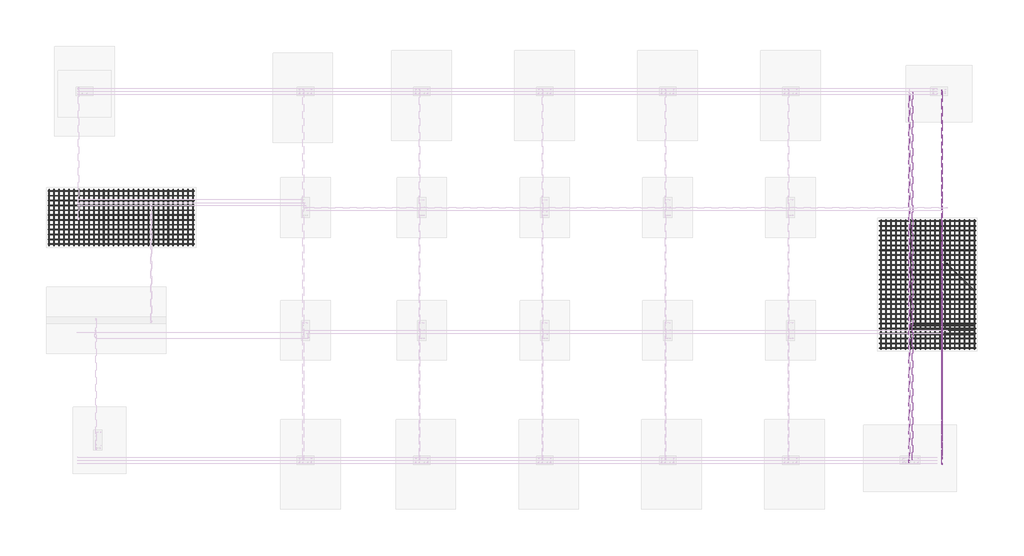
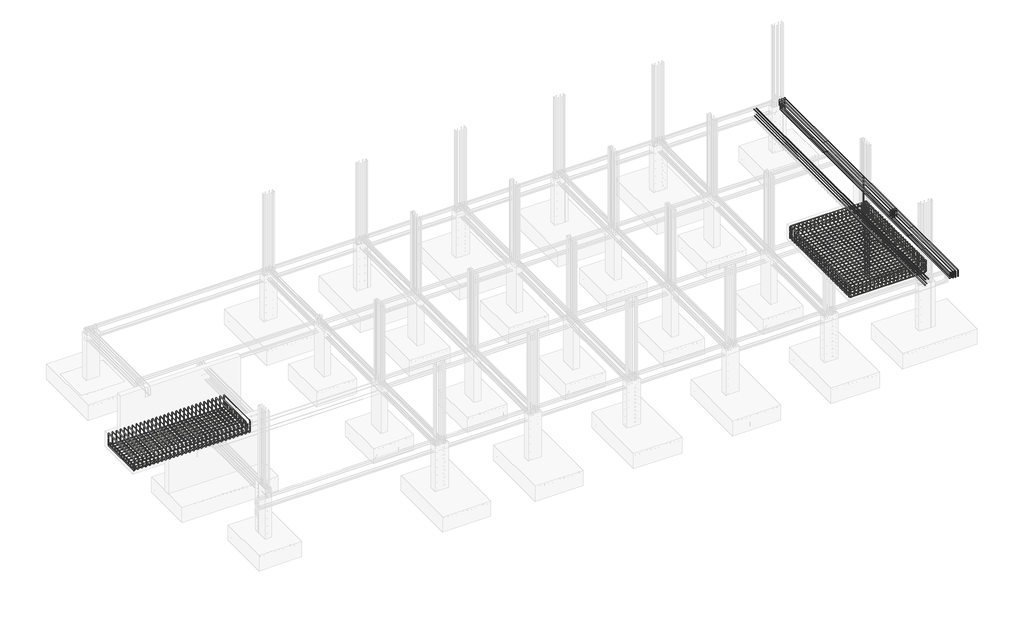
# One storey, part 10 of 18: 15 reinforcing bars.
"""IFC4 building model written with IfcOpenShell, lengths in millimetres."""

from ifc_helpers import new_model, si_unit, point, frame, origin, place, context, project, spatial, polyline, circle_curve, trimmed, segment, composite_curve, source, transform, mapped, element, save
from ifc_brep_helpers import swept_disk

model = new_model("IFC4")

# Units and contexts
model_context = context("Model", 3, world=origin())
ifc_project = project(units=[si_unit("LENGTHUNIT", "METRE", prefix="MILLI")], contexts=[model_context])

# Site, building, storey
site = spatial("IfcSite", under=ifc_project)
building = spatial("IfcBuilding", under=site)
storey = spatial("IfcBuildingStorey", under=building, Elevation=-2000.0)

# Reinforcing bars
placement = place(None, origin())
reinforcing_bar_shape = source(origin(), model_context, "Body", "SolidModel", [
    swept_disk(composite_curve([segment(polyline([(11487.920951, 1646.2024102, -2300.0), (11487.920951, 1646.2024102, -2486.6)]), True, "CONTINUOUS"), segment(trimmed(circle_curve(frame((11432.470951, 1646.2024102, -2486.6), z_axis=(0.0, 1.0, 0.0), x_axis=(55.45000000000073, 0.0, 0.0)), 55.45), [point((11487.920951, 1646.2024102, -2486.6))], [point((11432.470951, 1646.2024102, -2542.05))], True, "CARTESIAN"), True, "CONTINUOUS"), segment(polyline([(11432.470951, 1646.2024102, -2542.05), (8659.270951, 1646.2024102, -2542.05)]), True, "CONTINUOUS"), segment(trimmed(circle_curve(frame((8659.270951, 1646.2024102, -2486.6), z_axis=(0.0, 1.0, 0.0), x_axis=(0.0, 0.0, -55.45000000000027)), 55.45), [point((8659.270951, 1646.2024102, -2542.05))], [point((8603.820951, 1646.2024102, -2486.6))], True, "CARTESIAN"), True, "CONTINUOUS"), segment(polyline([(8603.820951, 1646.2024102, -2486.6), (8603.820951, 1646.2024102, -2300.0)]), True, "CONTINUOUS")], self_intersect=False), 7.95),
])
element("IfcReinforcingBar", 1, at=placement, inside=storey, context=model_context, shape_type="MappedRepresentation", body=[
    mapped(reinforcing_bar_shape, transform((0.0, 0.0, 0.0), x_axis=(1.0, 0.0, 0.0), y_axis=(0.0, 1.0, 0.0), z_axis=(0.0, 0.0, 1.0))),
    mapped(reinforcing_bar_shape, transform((0.0, -147.4106069, 0.0), x_axis=(1.0, 0.0, 0.0), y_axis=(0.0, 1.0, 0.0), z_axis=(0.0, 0.0, 1.0))),
    mapped(reinforcing_bar_shape, transform((0.0, -294.8212138, 0.0), x_axis=(1.0, 0.0, 0.0), y_axis=(0.0, 1.0, 0.0), z_axis=(0.0, 0.0, 1.0))),
    mapped(reinforcing_bar_shape, transform((0.0, -442.2318207, 0.0), x_axis=(1.0, 0.0, 0.0), y_axis=(0.0, 1.0, 0.0), z_axis=(0.0, 0.0, 1.0))),
    mapped(reinforcing_bar_shape, transform((0.0, -589.6424276, 0.0), x_axis=(1.0, 0.0, 0.0), y_axis=(0.0, 1.0, 0.0), z_axis=(0.0, 0.0, 1.0))),
    mapped(reinforcing_bar_shape, transform((0.0, -737.0530345, 0.0), x_axis=(1.0, 0.0, 0.0), y_axis=(0.0, 1.0, 0.0), z_axis=(0.0, 0.0, 1.0))),
    mapped(reinforcing_bar_shape, transform((0.0, -884.4636415, 0.0), x_axis=(1.0, 0.0, 0.0), y_axis=(0.0, 1.0, 0.0), z_axis=(0.0, 0.0, 1.0))),
    mapped(reinforcing_bar_shape, transform((0.0, -1031.8742484, 0.0), x_axis=(1.0, 0.0, 0.0), y_axis=(0.0, 1.0, 0.0), z_axis=(0.0, 0.0, 1.0))),
    mapped(reinforcing_bar_shape, transform((0.0, -1179.2848553, 0.0), x_axis=(1.0, 0.0, 0.0), y_axis=(0.0, 1.0, 0.0), z_axis=(0.0, 0.0, 1.0))),
    mapped(reinforcing_bar_shape, transform((0.0, -1326.6954622, 0.0), x_axis=(1.0, 0.0, 0.0), y_axis=(0.0, 1.0, 0.0), z_axis=(0.0, 0.0, 1.0))),
    mapped(reinforcing_bar_shape, transform((0.0, -1474.1060691, 0.0), x_axis=(1.0, 0.0, 0.0), y_axis=(0.0, 1.0, 0.0), z_axis=(0.0, 0.0, 1.0))),
    mapped(reinforcing_bar_shape, transform((0.0, -1621.516676, 0.0), x_axis=(1.0, 0.0, 0.0), y_axis=(0.0, 1.0, 0.0), z_axis=(0.0, 0.0, 1.0))),
    mapped(reinforcing_bar_shape, transform((0.0, -1768.9272829, 0.0), x_axis=(1.0, 0.0, 0.0), y_axis=(0.0, 1.0, 0.0), z_axis=(0.0, 0.0, 1.0))),
    mapped(reinforcing_bar_shape, transform((0.0, -1916.3378898, 0.0), x_axis=(1.0, 0.0, 0.0), y_axis=(0.0, 1.0, 0.0), z_axis=(0.0, 0.0, 1.0))),
    mapped(reinforcing_bar_shape, transform((0.0, -2063.7484967, 0.0), x_axis=(1.0, 0.0, 0.0), y_axis=(0.0, 1.0, 0.0), z_axis=(0.0, 0.0, 1.0))),
    mapped(reinforcing_bar_shape, transform((0.0, -2211.1591036, 0.0), x_axis=(1.0, 0.0, 0.0), y_axis=(0.0, 1.0, 0.0), z_axis=(0.0, 0.0, 1.0))),
    mapped(reinforcing_bar_shape, transform((0.0, -2358.5697105, 0.0), x_axis=(1.0, 0.0, 0.0), y_axis=(0.0, 1.0, 0.0), z_axis=(0.0, 0.0, 1.0))),
    mapped(reinforcing_bar_shape, transform((0.0, -2505.9803174, 0.0), x_axis=(1.0, 0.0, 0.0), y_axis=(0.0, 1.0, 0.0), z_axis=(0.0, 0.0, 1.0))),
    mapped(reinforcing_bar_shape, transform((0.0, -2653.3909244, 0.0), x_axis=(1.0, 0.0, 0.0), y_axis=(0.0, 1.0, 0.0), z_axis=(0.0, 0.0, 1.0))),
    mapped(reinforcing_bar_shape, transform((0.0, -2800.8015313, 0.0), x_axis=(1.0, 0.0, 0.0), y_axis=(0.0, 1.0, 0.0), z_axis=(0.0, 0.0, 1.0))),
    mapped(reinforcing_bar_shape, transform((0.0, -2948.2121382, 0.0), x_axis=(1.0, 0.0, 0.0), y_axis=(0.0, 1.0, 0.0), z_axis=(0.0, 0.0, 1.0))),
    mapped(reinforcing_bar_shape, transform((0.0, -3095.6227451, 0.0), x_axis=(1.0, 0.0, 0.0), y_axis=(0.0, 1.0, 0.0), z_axis=(0.0, 0.0, 1.0))),
    mapped(reinforcing_bar_shape, transform((0.0, -3243.033352, 0.0), x_axis=(1.0, 0.0, 0.0), y_axis=(0.0, 1.0, 0.0), z_axis=(0.0, 0.0, 1.0))),
    mapped(reinforcing_bar_shape, transform((0.0, -3390.4439589, 0.0), x_axis=(1.0, 0.0, 0.0), y_axis=(0.0, 1.0, 0.0), z_axis=(0.0, 0.0, 1.0))),
    mapped(reinforcing_bar_shape, transform((0.0, -3537.8545658, 0.0), x_axis=(1.0, 0.0, 0.0), y_axis=(0.0, 1.0, 0.0), z_axis=(0.0, 0.0, 1.0))),
    mapped(reinforcing_bar_shape, transform((0.0, -3685.2651727, 0.0), x_axis=(1.0, 0.0, 0.0), y_axis=(0.0, 1.0, 0.0), z_axis=(0.0, 0.0, 1.0))),
    mapped(reinforcing_bar_shape, transform((0.0, -3832.6757796, 0.0), x_axis=(1.0, 0.0, 0.0), y_axis=(0.0, 1.0, 0.0), z_axis=(0.0, 0.0, 1.0))),
])
reinforcing_bar_2_shape = source(origin(), model_context, "Body", "SolidModel", [
    swept_disk(composite_curve([segment(polyline([(8601.870951, 1646.2024102, -2250.0), (8601.870951, 1646.2024102, -2102.0)]), True, "CONTINUOUS"), segment(trimmed(circle_curve(frame((8647.870951, 1646.2024102, -2102.0), z_axis=(0.0, 1.0, 0.0), x_axis=(-46.0, 0.0, 0.0)), 46.0), [point((8601.870951, 1646.2024102, -2102.0))], [point((8647.870951, 1646.2024102, -2056.0))], True, "CARTESIAN"), True, "CONTINUOUS"), segment(polyline([(8647.870951, 1646.2024102, -2056.0), (11443.870951, 1646.2024102, -2056.0)]), True, "CONTINUOUS"), segment(trimmed(circle_curve(frame((11443.870951, 1646.2024102, -2102.0), z_axis=(0.0, 1.0, 0.0), x_axis=(0.0, 0.0, 46.0)), 46.0), [point((11443.870951, 1646.2024102, -2056.0))], [point((11489.870951, 1646.2024102, -2102.0))], True, "CARTESIAN"), True, "CONTINUOUS"), segment(polyline([(11489.870951, 1646.2024102, -2102.0), (11489.870951, 1646.2024102, -2250.0)]), True, "CONTINUOUS")], self_intersect=False), 6.0),
])
element("IfcReinforcingBar", 2, at=placement, inside=storey, context=model_context, shape_type="MappedRepresentation", body=[
    mapped(reinforcing_bar_2_shape, transform((0.0, 0.0, 0.0), x_axis=(1.0, 0.0, 0.0), y_axis=(0.0, 1.0, 0.0), z_axis=(0.0, 0.0, 1.0))),
    mapped(reinforcing_bar_2_shape, transform((0.0, -147.4106069, 0.0), x_axis=(1.0, 0.0, 0.0), y_axis=(0.0, 1.0, 0.0), z_axis=(0.0, 0.0, 1.0))),
    mapped(reinforcing_bar_2_shape, transform((0.0, -294.8212138, 0.0), x_axis=(1.0, 0.0, 0.0), y_axis=(0.0, 1.0, 0.0), z_axis=(0.0, 0.0, 1.0))),
    mapped(reinforcing_bar_2_shape, transform((0.0, -442.2318207, 0.0), x_axis=(1.0, 0.0, 0.0), y_axis=(0.0, 1.0, 0.0), z_axis=(0.0, 0.0, 1.0))),
    mapped(reinforcing_bar_2_shape, transform((0.0, -589.6424276, 0.0), x_axis=(1.0, 0.0, 0.0), y_axis=(0.0, 1.0, 0.0), z_axis=(0.0, 0.0, 1.0))),
    mapped(reinforcing_bar_2_shape, transform((0.0, -737.0530345, 0.0), x_axis=(1.0, 0.0, 0.0), y_axis=(0.0, 1.0, 0.0), z_axis=(0.0, 0.0, 1.0))),
    mapped(reinforcing_bar_2_shape, transform((0.0, -884.4636415, 0.0), x_axis=(1.0, 0.0, 0.0), y_axis=(0.0, 1.0, 0.0), z_axis=(0.0, 0.0, 1.0))),
    mapped(reinforcing_bar_2_shape, transform((0.0, -1031.8742484, 0.0), x_axis=(1.0, 0.0, 0.0), y_axis=(0.0, 1.0, 0.0), z_axis=(0.0, 0.0, 1.0))),
    mapped(reinforcing_bar_2_shape, transform((0.0, -1179.2848553, 0.0), x_axis=(1.0, 0.0, 0.0), y_axis=(0.0, 1.0, 0.0), z_axis=(0.0, 0.0, 1.0))),
    mapped(reinforcing_bar_2_shape, transform((0.0, -1326.6954622, 0.0), x_axis=(1.0, 0.0, 0.0), y_axis=(0.0, 1.0, 0.0), z_axis=(0.0, 0.0, 1.0))),
    mapped(reinforcing_bar_2_shape, transform((0.0, -1474.1060691, 0.0), x_axis=(1.0, 0.0, 0.0), y_axis=(0.0, 1.0, 0.0), z_axis=(0.0, 0.0, 1.0))),
    mapped(reinforcing_bar_2_shape, transform((0.0, -1621.516676, 0.0), x_axis=(1.0, 0.0, 0.0), y_axis=(0.0, 1.0, 0.0), z_axis=(0.0, 0.0, 1.0))),
    mapped(reinforcing_bar_2_shape, transform((0.0, -1768.9272829, 0.0), x_axis=(1.0, 0.0, 0.0), y_axis=(0.0, 1.0, 0.0), z_axis=(0.0, 0.0, 1.0))),
    mapped(reinforcing_bar_2_shape, transform((0.0, -1916.3378898, 0.0), x_axis=(1.0, 0.0, 0.0), y_axis=(0.0, 1.0, 0.0), z_axis=(0.0, 0.0, 1.0))),
    mapped(reinforcing_bar_2_shape, transform((0.0, -2063.7484967, 0.0), x_axis=(1.0, 0.0, 0.0), y_axis=(0.0, 1.0, 0.0), z_axis=(0.0, 0.0, 1.0))),
    mapped(reinforcing_bar_2_shape, transform((0.0, -2211.1591036, 0.0), x_axis=(1.0, 0.0, 0.0), y_axis=(0.0, 1.0, 0.0), z_axis=(0.0, 0.0, 1.0))),
    mapped(reinforcing_bar_2_shape, transform((0.0, -2358.5697105, 0.0), x_axis=(1.0, 0.0, 0.0), y_axis=(0.0, 1.0, 0.0), z_axis=(0.0, 0.0, 1.0))),
    mapped(reinforcing_bar_2_shape, transform((0.0, -2505.9803174, 0.0), x_axis=(1.0, 0.0, 0.0), y_axis=(0.0, 1.0, 0.0), z_axis=(0.0, 0.0, 1.0))),
    mapped(reinforcing_bar_2_shape, transform((0.0, -2653.3909244, 0.0), x_axis=(1.0, 0.0, 0.0), y_axis=(0.0, 1.0, 0.0), z_axis=(0.0, 0.0, 1.0))),
    mapped(reinforcing_bar_2_shape, transform((0.0, -2800.8015313, 0.0), x_axis=(1.0, 0.0, 0.0), y_axis=(0.0, 1.0, 0.0), z_axis=(0.0, 0.0, 1.0))),
    mapped(reinforcing_bar_2_shape, transform((0.0, -2948.2121382, 0.0), x_axis=(1.0, 0.0, 0.0), y_axis=(0.0, 1.0, 0.0), z_axis=(0.0, 0.0, 1.0))),
    mapped(reinforcing_bar_2_shape, transform((0.0, -3095.6227451, 0.0), x_axis=(1.0, 0.0, 0.0), y_axis=(0.0, 1.0, 0.0), z_axis=(0.0, 0.0, 1.0))),
    mapped(reinforcing_bar_2_shape, transform((0.0, -3243.033352, 0.0), x_axis=(1.0, 0.0, 0.0), y_axis=(0.0, 1.0, 0.0), z_axis=(0.0, 0.0, 1.0))),
    mapped(reinforcing_bar_2_shape, transform((0.0, -3390.4439589, 0.0), x_axis=(1.0, 0.0, 0.0), y_axis=(0.0, 1.0, 0.0), z_axis=(0.0, 0.0, 1.0))),
    mapped(reinforcing_bar_2_shape, transform((0.0, -3537.8545658, 0.0), x_axis=(1.0, 0.0, 0.0), y_axis=(0.0, 1.0, 0.0), z_axis=(0.0, 0.0, 1.0))),
    mapped(reinforcing_bar_2_shape, transform((0.0, -3685.2651727, 0.0), x_axis=(1.0, 0.0, 0.0), y_axis=(0.0, 1.0, 0.0), z_axis=(0.0, 0.0, 1.0))),
    mapped(reinforcing_bar_2_shape, transform((0.0, -3832.6757796, 0.0), x_axis=(1.0, 0.0, 0.0), y_axis=(0.0, 1.0, 0.0), z_axis=(0.0, 0.0, 1.0))),
])
reinforcing_bar_3_shape = source(origin(), model_context, "Body", "SolidModel", [
    swept_disk(composite_curve([segment(polyline([(8648.0517338, 1669.0978854, -2322.6684255), (8648.0517338, 1669.0978854, -2470.6684255)]), True, "CONTINUOUS"), segment(trimmed(circle_curve(frame((8648.0517338, 1623.0978854, -2470.6684255), z_axis=(-1.0, 0.0, 0.0), x_axis=(0.0, 46.0, 0.0)), 46.0), [point((8648.0517338, 1669.0978854, -2470.6684255))], [point((8648.0517338, 1623.0978854, -2516.6684255))], True, "CARTESIAN"), True, "CONTINUOUS"), segment(polyline([(8648.0517338, 1623.0978854, -2516.6684255), (8648.0517338, -2172.9021146, -2516.6684255)]), True, "CONTINUOUS"), segment(trimmed(circle_curve(frame((8648.0517338, -2172.9021146, -2470.6684255), z_axis=(-1.0, 0.0, 0.0), x_axis=(0.0, 0.0, -46.0)), 46.0), [point((8648.0517338, -2172.9021146, -2516.6684255))], [point((8648.0517338, -2218.9021146, -2470.6684255))], True, "CARTESIAN"), True, "CONTINUOUS"), segment(polyline([(8648.0517338, -2218.9021146, -2470.6684255), (8648.0517338, -2218.9021146, -2322.6684255)]), True, "CONTINUOUS")], self_intersect=False), 6.0),
])
element("IfcReinforcingBar", 3, at=placement, inside=storey, context=model_context, shape_type="MappedRepresentation", body=[
    mapped(reinforcing_bar_3_shape, transform((0.0, 0.0, 0.0), x_axis=(1.0, 0.0, 0.0), y_axis=(0.0, 1.0, 0.0), z_axis=(0.0, 0.0, 1.0))),
    mapped(reinforcing_bar_3_shape, transform((147.5694243, 0.0, 0.0), x_axis=(1.0, 0.0, 0.0), y_axis=(0.0, 1.0, 0.0), z_axis=(0.0, 0.0, 1.0))),
    mapped(reinforcing_bar_3_shape, transform((295.1388487, 0.0, 0.0), x_axis=(1.0, 0.0, 0.0), y_axis=(0.0, 1.0, 0.0), z_axis=(0.0, 0.0, 1.0))),
    mapped(reinforcing_bar_3_shape, transform((442.708273, 0.0, 0.0), x_axis=(1.0, 0.0, 0.0), y_axis=(0.0, 1.0, 0.0), z_axis=(0.0, 0.0, 1.0))),
    mapped(reinforcing_bar_3_shape, transform((590.2776973, 0.0, 0.0), x_axis=(1.0, 0.0, 0.0), y_axis=(0.0, 1.0, 0.0), z_axis=(0.0, 0.0, 1.0))),
    mapped(reinforcing_bar_3_shape, transform((737.8471217, 0.0, 0.0), x_axis=(1.0, 0.0, 0.0), y_axis=(0.0, 1.0, 0.0), z_axis=(0.0, 0.0, 1.0))),
    mapped(reinforcing_bar_3_shape, transform((885.416546, 0.0, 0.0), x_axis=(1.0, 0.0, 0.0), y_axis=(0.0, 1.0, 0.0), z_axis=(0.0, 0.0, 1.0))),
    mapped(reinforcing_bar_3_shape, transform((1032.9859703, 0.0, 0.0), x_axis=(1.0, 0.0, 0.0), y_axis=(0.0, 1.0, 0.0), z_axis=(0.0, 0.0, 1.0))),
    mapped(reinforcing_bar_3_shape, transform((1180.5553947, 0.0, 0.0), x_axis=(1.0, 0.0, 0.0), y_axis=(0.0, 1.0, 0.0), z_axis=(0.0, 0.0, 1.0))),
    mapped(reinforcing_bar_3_shape, transform((1328.124819, 0.0, 0.0), x_axis=(1.0, 0.0, 0.0), y_axis=(0.0, 1.0, 0.0), z_axis=(0.0, 0.0, 1.0))),
    mapped(reinforcing_bar_3_shape, transform((1475.6942433, 0.0, 0.0), x_axis=(1.0, 0.0, 0.0), y_axis=(0.0, 1.0, 0.0), z_axis=(0.0, 0.0, 1.0))),
    mapped(reinforcing_bar_3_shape, transform((1623.2636677, 0.0, 0.0), x_axis=(1.0, 0.0, 0.0), y_axis=(0.0, 1.0, 0.0), z_axis=(0.0, 0.0, 1.0))),
    mapped(reinforcing_bar_3_shape, transform((1770.833092, 0.0, 0.0), x_axis=(1.0, 0.0, 0.0), y_axis=(0.0, 1.0, 0.0), z_axis=(0.0, 0.0, 1.0))),
    mapped(reinforcing_bar_3_shape, transform((1918.4025163, 0.0, 0.0), x_axis=(1.0, 0.0, 0.0), y_axis=(0.0, 1.0, 0.0), z_axis=(0.0, 0.0, 1.0))),
    mapped(reinforcing_bar_3_shape, transform((2065.9719407, 0.0, 0.0), x_axis=(1.0, 0.0, 0.0), y_axis=(0.0, 1.0, 0.0), z_axis=(0.0, 0.0, 1.0))),
    mapped(reinforcing_bar_3_shape, transform((2213.541365, 0.0, 0.0), x_axis=(1.0, 0.0, 0.0), y_axis=(0.0, 1.0, 0.0), z_axis=(0.0, 0.0, 1.0))),
    mapped(reinforcing_bar_3_shape, transform((2361.1107893, 0.0, 0.0), x_axis=(1.0, 0.0, 0.0), y_axis=(0.0, 1.0, 0.0), z_axis=(0.0, 0.0, 1.0))),
    mapped(reinforcing_bar_3_shape, transform((2508.6802137, 0.0, 0.0), x_axis=(1.0, 0.0, 0.0), y_axis=(0.0, 1.0, 0.0), z_axis=(0.0, 0.0, 1.0))),
    mapped(reinforcing_bar_3_shape, transform((2656.249638, 0.0, 0.0), x_axis=(1.0, 0.0, 0.0), y_axis=(0.0, 1.0, 0.0), z_axis=(0.0, 0.0, 1.0))),
    mapped(reinforcing_bar_3_shape, transform((2803.8190623, 0.0, 0.0), x_axis=(1.0, 0.0, 0.0), y_axis=(0.0, 1.0, 0.0), z_axis=(0.0, 0.0, 1.0))),
])
reinforcing_bar_4_shape = source(origin(), model_context, "Body", "SolidModel", [
    swept_disk(composite_curve([segment(polyline([(11453.793968, 1669.0978854, -2276.6677805), (11453.793968, 1669.0978854, -2128.6677805)]), True, "CONTINUOUS"), segment(trimmed(circle_curve(frame((11453.793968, 1623.0978854, -2128.6677805), z_axis=(1.0, 0.0, 0.0), x_axis=(0.0, 46.0, 0.0)), 46.0), [point((11453.793968, 1669.0978854, -2128.6677805))], [point((11453.793968, 1623.0978854, -2082.6677805))], True, "CARTESIAN"), True, "CONTINUOUS"), segment(polyline([(11453.793968, 1623.0978854, -2082.6677805), (11453.793968, -2172.9021146, -2082.6677805)]), True, "CONTINUOUS"), segment(trimmed(circle_curve(frame((11453.793968, -2172.9021146, -2128.6677805), z_axis=(1.0, 0.0, 0.0), x_axis=(0.0, 0.0, 46.0)), 46.0), [point((11453.793968, -2172.9021146, -2082.6677805))], [point((11453.793968, -2218.9021146, -2128.6677805))], True, "CARTESIAN"), True, "CONTINUOUS"), segment(polyline([(11453.793968, -2218.9021146, -2128.6677805), (11453.793968, -2218.9021146, -2276.6677805)]), True, "CONTINUOUS")], self_intersect=False), 6.0),
])
element("IfcReinforcingBar", 4, at=placement, inside=storey, context=model_context, shape_type="MappedRepresentation", body=[
    mapped(reinforcing_bar_4_shape, transform((0.0, 0.0, 0.0), x_axis=(1.0, 0.0, 0.0), y_axis=(0.0, 1.0, 0.0), z_axis=(0.0, 0.0, 1.0))),
    mapped(reinforcing_bar_4_shape, transform((-147.6706439, 0.0, 0.0), x_axis=(1.0, 0.0, 0.0), y_axis=(0.0, 1.0, 0.0), z_axis=(0.0, 0.0, 1.0))),
    mapped(reinforcing_bar_4_shape, transform((-295.3412878, 0.0, 0.0), x_axis=(1.0, 0.0, 0.0), y_axis=(0.0, 1.0, 0.0), z_axis=(0.0, 0.0, 1.0))),
    mapped(reinforcing_bar_4_shape, transform((-443.0119317, 0.0, 0.0), x_axis=(1.0, 0.0, 0.0), y_axis=(0.0, 1.0, 0.0), z_axis=(0.0, 0.0, 1.0))),
    mapped(reinforcing_bar_4_shape, transform((-590.6825756, 0.0, 0.0), x_axis=(1.0, 0.0, 0.0), y_axis=(0.0, 1.0, 0.0), z_axis=(0.0, 0.0, 1.0))),
    mapped(reinforcing_bar_4_shape, transform((-738.3532195, 0.0, 0.0), x_axis=(1.0, 0.0, 0.0), y_axis=(0.0, 1.0, 0.0), z_axis=(0.0, 0.0, 1.0))),
    mapped(reinforcing_bar_4_shape, transform((-886.0238634, 0.0, 0.0), x_axis=(1.0, 0.0, 0.0), y_axis=(0.0, 1.0, 0.0), z_axis=(0.0, 0.0, 1.0))),
    mapped(reinforcing_bar_4_shape, transform((-1033.6945073, 0.0, 0.0), x_axis=(1.0, 0.0, 0.0), y_axis=(0.0, 1.0, 0.0), z_axis=(0.0, 0.0, 1.0))),
    mapped(reinforcing_bar_4_shape, transform((-1181.3651512, 0.0, 0.0), x_axis=(1.0, 0.0, 0.0), y_axis=(0.0, 1.0, 0.0), z_axis=(0.0, 0.0, 1.0))),
    mapped(reinforcing_bar_4_shape, transform((-1329.0357951, 0.0, 0.0), x_axis=(1.0, 0.0, 0.0), y_axis=(0.0, 1.0, 0.0), z_axis=(0.0, 0.0, 1.0))),
    mapped(reinforcing_bar_4_shape, transform((-1476.706439, 0.0, 0.0), x_axis=(1.0, 0.0, 0.0), y_axis=(0.0, 1.0, 0.0), z_axis=(0.0, 0.0, 1.0))),
    mapped(reinforcing_bar_4_shape, transform((-1624.3770829, 0.0, 0.0), x_axis=(1.0, 0.0, 0.0), y_axis=(0.0, 1.0, 0.0), z_axis=(0.0, 0.0, 1.0))),
    mapped(reinforcing_bar_4_shape, transform((-1772.0477268, 0.0, 0.0), x_axis=(1.0, 0.0, 0.0), y_axis=(0.0, 1.0, 0.0), z_axis=(0.0, 0.0, 1.0))),
    mapped(reinforcing_bar_4_shape, transform((-1919.7183707, 0.0, 0.0), x_axis=(1.0, 0.0, 0.0), y_axis=(0.0, 1.0, 0.0), z_axis=(0.0, 0.0, 1.0))),
    mapped(reinforcing_bar_4_shape, transform((-2067.3890146, 0.0, 0.0), x_axis=(1.0, 0.0, 0.0), y_axis=(0.0, 1.0, 0.0), z_axis=(0.0, 0.0, 1.0))),
    mapped(reinforcing_bar_4_shape, transform((-2215.0596586, 0.0, 0.0), x_axis=(1.0, 0.0, 0.0), y_axis=(0.0, 1.0, 0.0), z_axis=(0.0, 0.0, 1.0))),
    mapped(reinforcing_bar_4_shape, transform((-2362.7303025, 0.0, 0.0), x_axis=(1.0, 0.0, 0.0), y_axis=(0.0, 1.0, 0.0), z_axis=(0.0, 0.0, 1.0))),
    mapped(reinforcing_bar_4_shape, transform((-2510.4009464, 0.0, 0.0), x_axis=(1.0, 0.0, 0.0), y_axis=(0.0, 1.0, 0.0), z_axis=(0.0, 0.0, 1.0))),
    mapped(reinforcing_bar_4_shape, transform((-2658.0715903, 0.0, 0.0), x_axis=(1.0, 0.0, 0.0), y_axis=(0.0, 1.0, 0.0), z_axis=(0.0, 0.0, 1.0))),
    mapped(reinforcing_bar_4_shape, transform((-2805.7422342, 0.0, 0.0), x_axis=(1.0, 0.0, 0.0), y_axis=(0.0, 1.0, 0.0), z_axis=(0.0, 0.0, 1.0))),
])
reinforcing_bar_5_shape = source(origin(), model_context, "Body", "SolidModel", [
    swept_disk(composite_curve([segment(polyline([(-16391.7002589, 2584.6478854, -2300.0), (-16391.7002589, 2584.6478854, -2486.6)]), True, "CONTINUOUS"), segment(trimmed(circle_curve(frame((-16391.7002589, 2529.1978854, -2486.6), z_axis=(-1.0, 0.0, 0.0), x_axis=(0.0, 55.45000000000027, 0.0)), 55.45), [point((-16391.7002589, 2584.6478854, -2486.6))], [point((-16391.7002589, 2529.1978854, -2542.05))], True, "CARTESIAN"), True, "CONTINUOUS"), segment(polyline([(-16391.7002589, 2529.1978854, -2542.05), (-16391.7002589, 955.9978854, -2542.05)]), True, "CONTINUOUS"), segment(trimmed(circle_curve(frame((-16391.7002589, 955.9978854, -2486.6), z_axis=(-1.0, 0.0, 0.0), x_axis=(0.0, 0.0, -55.45000000000027)), 55.45), [point((-16391.7002589, 955.9978854, -2542.05))], [point((-16391.7002589, 900.5478854, -2486.6))], True, "CARTESIAN"), True, "CONTINUOUS"), segment(polyline([(-16391.7002589, 900.5478854, -2486.6), (-16391.7002589, 900.5478854, -2300.0)]), True, "CONTINUOUS")], self_intersect=False), 7.95),
])
element("IfcReinforcingBar", 5, at=placement, inside=storey, context=model_context, shape_type="MappedRepresentation", body=[
    mapped(reinforcing_bar_5_shape, transform((0.0, 0.0, 0.0), x_axis=(1.0, 0.0, 0.0), y_axis=(0.0, 1.0, 0.0), z_axis=(0.0, 0.0, 1.0))),
    mapped(reinforcing_bar_5_shape, transform((149.3336476, 0.0, 0.0), x_axis=(1.0, 0.0, 0.0), y_axis=(0.0, 1.0, 0.0), z_axis=(0.0, 0.0, 1.0))),
    mapped(reinforcing_bar_5_shape, transform((298.6672951, 0.0, 0.0), x_axis=(1.0, 0.0, 0.0), y_axis=(0.0, 1.0, 0.0), z_axis=(0.0, 0.0, 1.0))),
    mapped(reinforcing_bar_5_shape, transform((448.0009427, 0.0, 0.0), x_axis=(1.0, 0.0, 0.0), y_axis=(0.0, 1.0, 0.0), z_axis=(0.0, 0.0, 1.0))),
    mapped(reinforcing_bar_5_shape, transform((597.3345903, 0.0, 0.0), x_axis=(1.0, 0.0, 0.0), y_axis=(0.0, 1.0, 0.0), z_axis=(0.0, 0.0, 1.0))),
    mapped(reinforcing_bar_5_shape, transform((746.6682379, 0.0, 0.0), x_axis=(1.0, 0.0, 0.0), y_axis=(0.0, 1.0, 0.0), z_axis=(0.0, 0.0, 1.0))),
    mapped(reinforcing_bar_5_shape, transform((896.0018854, 0.0, 0.0), x_axis=(1.0, 0.0, 0.0), y_axis=(0.0, 1.0, 0.0), z_axis=(0.0, 0.0, 1.0))),
    mapped(reinforcing_bar_5_shape, transform((1045.335533, 0.0, 0.0), x_axis=(1.0, 0.0, 0.0), y_axis=(0.0, 1.0, 0.0), z_axis=(0.0, 0.0, 1.0))),
    mapped(reinforcing_bar_5_shape, transform((1194.6691806, 0.0, 0.0), x_axis=(1.0, 0.0, 0.0), y_axis=(0.0, 1.0, 0.0), z_axis=(0.0, 0.0, 1.0))),
    mapped(reinforcing_bar_5_shape, transform((1344.0028282, 0.0, 0.0), x_axis=(1.0, 0.0, 0.0), y_axis=(0.0, 1.0, 0.0), z_axis=(0.0, 0.0, 1.0))),
    mapped(reinforcing_bar_5_shape, transform((1493.3364757, 0.0, 0.0), x_axis=(1.0, 0.0, 0.0), y_axis=(0.0, 1.0, 0.0), z_axis=(0.0, 0.0, 1.0))),
    mapped(reinforcing_bar_5_shape, transform((1642.6701233, 0.0, 0.0), x_axis=(1.0, 0.0, 0.0), y_axis=(0.0, 1.0, 0.0), z_axis=(0.0, 0.0, 1.0))),
    mapped(reinforcing_bar_5_shape, transform((1792.0037709, 0.0, 0.0), x_axis=(1.0, 0.0, 0.0), y_axis=(0.0, 1.0, 0.0), z_axis=(0.0, 0.0, 1.0))),
    mapped(reinforcing_bar_5_shape, transform((1941.3374185, 0.0, 0.0), x_axis=(1.0, 0.0, 0.0), y_axis=(0.0, 1.0, 0.0), z_axis=(0.0, 0.0, 1.0))),
    mapped(reinforcing_bar_5_shape, transform((2090.671066, 0.0, 0.0), x_axis=(1.0, 0.0, 0.0), y_axis=(0.0, 1.0, 0.0), z_axis=(0.0, 0.0, 1.0))),
    mapped(reinforcing_bar_5_shape, transform((2240.0047136, 0.0, 0.0), x_axis=(1.0, 0.0, 0.0), y_axis=(0.0, 1.0, 0.0), z_axis=(0.0, 0.0, 1.0))),
    mapped(reinforcing_bar_5_shape, transform((2389.3383612, 0.0, 0.0), x_axis=(1.0, 0.0, 0.0), y_axis=(0.0, 1.0, 0.0), z_axis=(0.0, 0.0, 1.0))),
    mapped(reinforcing_bar_5_shape, transform((2538.6720087, 0.0, 0.0), x_axis=(1.0, 0.0, 0.0), y_axis=(0.0, 1.0, 0.0), z_axis=(0.0, 0.0, 1.0))),
    mapped(reinforcing_bar_5_shape, transform((2688.0056563, 0.0, 0.0), x_axis=(1.0, 0.0, 0.0), y_axis=(0.0, 1.0, 0.0), z_axis=(0.0, 0.0, 1.0))),
    mapped(reinforcing_bar_5_shape, transform((2837.3393039, 0.0, 0.0), x_axis=(1.0, 0.0, 0.0), y_axis=(0.0, 1.0, 0.0), z_axis=(0.0, 0.0, 1.0))),
    mapped(reinforcing_bar_5_shape, transform((2986.6729515, 0.0, 0.0), x_axis=(1.0, 0.0, 0.0), y_axis=(0.0, 1.0, 0.0), z_axis=(0.0, 0.0, 1.0))),
    mapped(reinforcing_bar_5_shape, transform((3136.006599, 0.0, 0.0), x_axis=(1.0, 0.0, 0.0), y_axis=(0.0, 1.0, 0.0), z_axis=(0.0, 0.0, 1.0))),
    mapped(reinforcing_bar_5_shape, transform((3285.3402466, 0.0, 0.0), x_axis=(1.0, 0.0, 0.0), y_axis=(0.0, 1.0, 0.0), z_axis=(0.0, 0.0, 1.0))),
    mapped(reinforcing_bar_5_shape, transform((3434.6738942, 0.0, 0.0), x_axis=(1.0, 0.0, 0.0), y_axis=(0.0, 1.0, 0.0), z_axis=(0.0, 0.0, 1.0))),
    mapped(reinforcing_bar_5_shape, transform((3584.0075418, 0.0, 0.0), x_axis=(1.0, 0.0, 0.0), y_axis=(0.0, 1.0, 0.0), z_axis=(0.0, 0.0, 1.0))),
    mapped(reinforcing_bar_5_shape, transform((3733.3411893, 0.0, 0.0), x_axis=(1.0, 0.0, 0.0), y_axis=(0.0, 1.0, 0.0), z_axis=(0.0, 0.0, 1.0))),
    mapped(reinforcing_bar_5_shape, transform((3882.6748369, 0.0, 0.0), x_axis=(1.0, 0.0, 0.0), y_axis=(0.0, 1.0, 0.0), z_axis=(0.0, 0.0, 1.0))),
    mapped(reinforcing_bar_5_shape, transform((4032.0084845, 0.0, 0.0), x_axis=(1.0, 0.0, 0.0), y_axis=(0.0, 1.0, 0.0), z_axis=(0.0, 0.0, 1.0))),
    mapped(reinforcing_bar_5_shape, transform((4181.3421321, 0.0, 0.0), x_axis=(1.0, 0.0, 0.0), y_axis=(0.0, 1.0, 0.0), z_axis=(0.0, 0.0, 1.0))),
    mapped(reinforcing_bar_5_shape, transform((4330.6757796, 0.0, 0.0), x_axis=(1.0, 0.0, 0.0), y_axis=(0.0, 1.0, 0.0), z_axis=(0.0, 0.0, 1.0))),
])
reinforcing_bar_6_shape = source(origin(), model_context, "Body", "SolidModel", [
    swept_disk(composite_curve([segment(polyline([(-16391.7002589, 898.5978854, -2250.0), (-16391.7002589, 898.5978854, -2102.0)]), True, "CONTINUOUS"), segment(trimmed(circle_curve(frame((-16391.7002589, 944.5978854, -2102.0), z_axis=(-1.0, 0.0, 0.0), x_axis=(0.0, -46.0, 0.0)), 46.0), [point((-16391.7002589, 898.5978854, -2102.0))], [point((-16391.7002589, 944.5978854, -2056.0))], True, "CARTESIAN"), True, "CONTINUOUS"), segment(polyline([(-16391.7002589, 944.5978854, -2056.0), (-16391.7002589, 2540.5978854, -2056.0)]), True, "CONTINUOUS"), segment(trimmed(circle_curve(frame((-16391.7002589, 2540.5978854, -2102.0), z_axis=(-1.0, 0.0, 0.0), x_axis=(0.0, 0.0, 46.0)), 46.0), [point((-16391.7002589, 2540.5978854, -2056.0))], [point((-16391.7002589, 2586.5978854, -2102.0))], True, "CARTESIAN"), True, "CONTINUOUS"), segment(polyline([(-16391.7002589, 2586.5978854, -2102.0), (-16391.7002589, 2586.5978854, -2250.0)]), True, "CONTINUOUS")], self_intersect=False), 6.0),
])
element("IfcReinforcingBar", 6, at=placement, inside=storey, context=model_context, shape_type="MappedRepresentation", body=[
    mapped(reinforcing_bar_6_shape, transform((0.0, 0.0, 0.0), x_axis=(1.0, 0.0, 0.0), y_axis=(0.0, 1.0, 0.0), z_axis=(0.0, 0.0, 1.0))),
    mapped(reinforcing_bar_6_shape, transform((149.3336476, 0.0, 0.0), x_axis=(1.0, 0.0, 0.0), y_axis=(0.0, 1.0, 0.0), z_axis=(0.0, 0.0, 1.0))),
    mapped(reinforcing_bar_6_shape, transform((298.6672951, 0.0, 0.0), x_axis=(1.0, 0.0, 0.0), y_axis=(0.0, 1.0, 0.0), z_axis=(0.0, 0.0, 1.0))),
    mapped(reinforcing_bar_6_shape, transform((448.0009427, 0.0, 0.0), x_axis=(1.0, 0.0, 0.0), y_axis=(0.0, 1.0, 0.0), z_axis=(0.0, 0.0, 1.0))),
    mapped(reinforcing_bar_6_shape, transform((597.3345903, 0.0, 0.0), x_axis=(1.0, 0.0, 0.0), y_axis=(0.0, 1.0, 0.0), z_axis=(0.0, 0.0, 1.0))),
    mapped(reinforcing_bar_6_shape, transform((746.6682379, 0.0, 0.0), x_axis=(1.0, 0.0, 0.0), y_axis=(0.0, 1.0, 0.0), z_axis=(0.0, 0.0, 1.0))),
    mapped(reinforcing_bar_6_shape, transform((896.0018854, 0.0, 0.0), x_axis=(1.0, 0.0, 0.0), y_axis=(0.0, 1.0, 0.0), z_axis=(0.0, 0.0, 1.0))),
    mapped(reinforcing_bar_6_shape, transform((1045.335533, 0.0, 0.0), x_axis=(1.0, 0.0, 0.0), y_axis=(0.0, 1.0, 0.0), z_axis=(0.0, 0.0, 1.0))),
    mapped(reinforcing_bar_6_shape, transform((1194.6691806, 0.0, 0.0), x_axis=(1.0, 0.0, 0.0), y_axis=(0.0, 1.0, 0.0), z_axis=(0.0, 0.0, 1.0))),
    mapped(reinforcing_bar_6_shape, transform((1344.0028282, 0.0, 0.0), x_axis=(1.0, 0.0, 0.0), y_axis=(0.0, 1.0, 0.0), z_axis=(0.0, 0.0, 1.0))),
    mapped(reinforcing_bar_6_shape, transform((1493.3364757, 0.0, 0.0), x_axis=(1.0, 0.0, 0.0), y_axis=(0.0, 1.0, 0.0), z_axis=(0.0, 0.0, 1.0))),
    mapped(reinforcing_bar_6_shape, transform((1642.6701233, 0.0, 0.0), x_axis=(1.0, 0.0, 0.0), y_axis=(0.0, 1.0, 0.0), z_axis=(0.0, 0.0, 1.0))),
    mapped(reinforcing_bar_6_shape, transform((1792.0037709, 0.0, 0.0), x_axis=(1.0, 0.0, 0.0), y_axis=(0.0, 1.0, 0.0), z_axis=(0.0, 0.0, 1.0))),
    mapped(reinforcing_bar_6_shape, transform((1941.3374185, 0.0, 0.0), x_axis=(1.0, 0.0, 0.0), y_axis=(0.0, 1.0, 0.0), z_axis=(0.0, 0.0, 1.0))),
    mapped(reinforcing_bar_6_shape, transform((2090.671066, 0.0, 0.0), x_axis=(1.0, 0.0, 0.0), y_axis=(0.0, 1.0, 0.0), z_axis=(0.0, 0.0, 1.0))),
    mapped(reinforcing_bar_6_shape, transform((2240.0047136, 0.0, 0.0), x_axis=(1.0, 0.0, 0.0), y_axis=(0.0, 1.0, 0.0), z_axis=(0.0, 0.0, 1.0))),
    mapped(reinforcing_bar_6_shape, transform((2389.3383612, 0.0, 0.0), x_axis=(1.0, 0.0, 0.0), y_axis=(0.0, 1.0, 0.0), z_axis=(0.0, 0.0, 1.0))),
    mapped(reinforcing_bar_6_shape, transform((2538.6720087, 0.0, 0.0), x_axis=(1.0, 0.0, 0.0), y_axis=(0.0, 1.0, 0.0), z_axis=(0.0, 0.0, 1.0))),
    mapped(reinforcing_bar_6_shape, transform((2688.0056563, 0.0, 0.0), x_axis=(1.0, 0.0, 0.0), y_axis=(0.0, 1.0, 0.0), z_axis=(0.0, 0.0, 1.0))),
    mapped(reinforcing_bar_6_shape, transform((2837.3393039, 0.0, 0.0), x_axis=(1.0, 0.0, 0.0), y_axis=(0.0, 1.0, 0.0), z_axis=(0.0, 0.0, 1.0))),
    mapped(reinforcing_bar_6_shape, transform((2986.6729515, 0.0, 0.0), x_axis=(1.0, 0.0, 0.0), y_axis=(0.0, 1.0, 0.0), z_axis=(0.0, 0.0, 1.0))),
    mapped(reinforcing_bar_6_shape, transform((3136.006599, 0.0, 0.0), x_axis=(1.0, 0.0, 0.0), y_axis=(0.0, 1.0, 0.0), z_axis=(0.0, 0.0, 1.0))),
    mapped(reinforcing_bar_6_shape, transform((3285.3402466, 0.0, 0.0), x_axis=(1.0, 0.0, 0.0), y_axis=(0.0, 1.0, 0.0), z_axis=(0.0, 0.0, 1.0))),
    mapped(reinforcing_bar_6_shape, transform((3434.6738942, 0.0, 0.0), x_axis=(1.0, 0.0, 0.0), y_axis=(0.0, 1.0, 0.0), z_axis=(0.0, 0.0, 1.0))),
    mapped(reinforcing_bar_6_shape, transform((3584.0075418, 0.0, 0.0), x_axis=(1.0, 0.0, 0.0), y_axis=(0.0, 1.0, 0.0), z_axis=(0.0, 0.0, 1.0))),
    mapped(reinforcing_bar_6_shape, transform((3733.3411893, 0.0, 0.0), x_axis=(1.0, 0.0, 0.0), y_axis=(0.0, 1.0, 0.0), z_axis=(0.0, 0.0, 1.0))),
    mapped(reinforcing_bar_6_shape, transform((3882.6748369, 0.0, 0.0), x_axis=(1.0, 0.0, 0.0), y_axis=(0.0, 1.0, 0.0), z_axis=(0.0, 0.0, 1.0))),
    mapped(reinforcing_bar_6_shape, transform((4032.0084845, 0.0, 0.0), x_axis=(1.0, 0.0, 0.0), y_axis=(0.0, 1.0, 0.0), z_axis=(0.0, 0.0, 1.0))),
    mapped(reinforcing_bar_6_shape, transform((4181.3421321, 0.0, 0.0), x_axis=(1.0, 0.0, 0.0), y_axis=(0.0, 1.0, 0.0), z_axis=(0.0, 0.0, 1.0))),
    mapped(reinforcing_bar_6_shape, transform((4330.6757796, 0.0, 0.0), x_axis=(1.0, 0.0, 0.0), y_axis=(0.0, 1.0, 0.0), z_axis=(0.0, 0.0, 1.0))),
])
reinforcing_bar_7_shape = source(origin(), model_context, "Body", "SolidModel", [
    swept_disk(composite_curve([segment(polyline([(-16414.5957341, 944.7786683, -2322.6684255), (-16414.5957341, 944.7786683, -2470.6684255)]), True, "CONTINUOUS"), segment(trimmed(circle_curve(frame((-16368.5957341, 944.7786683, -2470.6684255), z_axis=(0.0, -1.0, 0.0), x_axis=(-46.0, 0.0, 0.0)), 46.0), [point((-16414.5957341, 944.7786683, -2470.6684255))], [point((-16368.5957341, 944.7786683, -2516.6684255))], True, "CARTESIAN"), True, "CONTINUOUS"), segment(polyline([(-16368.5957341, 944.7786683, -2516.6684255), (-12074.5957341, 944.7786683, -2516.6684255)]), True, "CONTINUOUS"), segment(trimmed(circle_curve(frame((-12074.5957341, 944.7786683, -2470.6684255), z_axis=(0.0, -1.0, 0.0), x_axis=(0.0, 0.0, -46.0)), 46.0), [point((-12074.5957341, 944.7786683, -2516.6684255))], [point((-12028.5957341, 944.7786683, -2470.6684255))], True, "CARTESIAN"), True, "CONTINUOUS"), segment(polyline([(-12028.5957341, 944.7786683, -2470.6684255), (-12028.5957341, 944.7786683, -2322.6684255)]), True, "CONTINUOUS")], self_intersect=False), 6.0),
])
element("IfcReinforcingBar", 7, at=placement, inside=storey, context=model_context, shape_type="MappedRepresentation", body=[
    mapped(reinforcing_bar_7_shape, transform((0.0, 0.0, 0.0), x_axis=(1.0, 0.0, 0.0), y_axis=(0.0, 1.0, 0.0), z_axis=(0.0, 0.0, 1.0))),
    mapped(reinforcing_bar_7_shape, transform((0.0, 145.8017329, 0.0), x_axis=(1.0, 0.0, 0.0), y_axis=(0.0, 1.0, 0.0), z_axis=(0.0, 0.0, 1.0))),
    mapped(reinforcing_bar_7_shape, transform((0.0, 291.6034659, 0.0), x_axis=(1.0, 0.0, 0.0), y_axis=(0.0, 1.0, 0.0), z_axis=(0.0, 0.0, 1.0))),
    mapped(reinforcing_bar_7_shape, transform((0.0, 437.4051988, 0.0), x_axis=(1.0, 0.0, 0.0), y_axis=(0.0, 1.0, 0.0), z_axis=(0.0, 0.0, 1.0))),
    mapped(reinforcing_bar_7_shape, transform((0.0, 583.2069318, 0.0), x_axis=(1.0, 0.0, 0.0), y_axis=(0.0, 1.0, 0.0), z_axis=(0.0, 0.0, 1.0))),
    mapped(reinforcing_bar_7_shape, transform((0.0, 729.0086647, 0.0), x_axis=(1.0, 0.0, 0.0), y_axis=(0.0, 1.0, 0.0), z_axis=(0.0, 0.0, 1.0))),
    mapped(reinforcing_bar_7_shape, transform((0.0, 874.8103976, 0.0), x_axis=(1.0, 0.0, 0.0), y_axis=(0.0, 1.0, 0.0), z_axis=(0.0, 0.0, 1.0))),
    mapped(reinforcing_bar_7_shape, transform((0.0, 1020.6121306, 0.0), x_axis=(1.0, 0.0, 0.0), y_axis=(0.0, 1.0, 0.0), z_axis=(0.0, 0.0, 1.0))),
    mapped(reinforcing_bar_7_shape, transform((0.0, 1166.4138635, 0.0), x_axis=(1.0, 0.0, 0.0), y_axis=(0.0, 1.0, 0.0), z_axis=(0.0, 0.0, 1.0))),
    mapped(reinforcing_bar_7_shape, transform((0.0, 1312.2155965, 0.0), x_axis=(1.0, 0.0, 0.0), y_axis=(0.0, 1.0, 0.0), z_axis=(0.0, 0.0, 1.0))),
    mapped(reinforcing_bar_7_shape, transform((0.0, 1458.0173294, 0.0), x_axis=(1.0, 0.0, 0.0), y_axis=(0.0, 1.0, 0.0), z_axis=(0.0, 0.0, 1.0))),
    mapped(reinforcing_bar_7_shape, transform((0.0, 1603.8190623, 0.0), x_axis=(1.0, 0.0, 0.0), y_axis=(0.0, 1.0, 0.0), z_axis=(0.0, 0.0, 1.0))),
])
reinforcing_bar_8_shape = source(origin(), model_context, "Body", "SolidModel", [
    swept_disk(composite_curve([segment(polyline([(9603.56265, -1776.5422299, -30.0), (9603.56265, -1776.5422299, -2436.6982733)]), True, "CONTINUOUS"), segment(trimmed(circle_curve(frame((9649.56265, -1776.5422299, -2436.6982733), z_axis=(0.0, -1.0, 0.0), x_axis=(-46.0, 0.0, 0.0)), 46.0), [point((9603.56265, -1776.5422299, -2436.6982733))], [point((9649.56265, -1776.5422299, -2482.6982733))], True, "CARTESIAN"), True, "CONTINUOUS"), segment(polyline([(9649.56265, -1776.5422299, -2482.6982733), (11445.1108185, -1776.5422299, -2482.6982733)]), True, "CONTINUOUS")], self_intersect=False), 6.0),
])
element("IfcReinforcingBar", 8, at=placement, inside=storey, context=model_context, shape_type="MappedRepresentation", body=[
    mapped(reinforcing_bar_8_shape, transform((0.0, 0.0, 0.0), x_axis=(1.0, 0.0, 0.0), y_axis=(0.0, 1.0, 0.0), z_axis=(0.0, 0.0, 1.0))),
    mapped(reinforcing_bar_8_shape, transform((0.0, 134.2724138, 0.0), x_axis=(1.0, 0.0, 0.0), y_axis=(0.0, 1.0, 0.0), z_axis=(0.0, 0.0, 1.0))),
    mapped(reinforcing_bar_8_shape, transform((0.0, 268.5448277, 0.0), x_axis=(1.0, 0.0, 0.0), y_axis=(0.0, 1.0, 0.0), z_axis=(0.0, 0.0, 1.0))),
])
element("IfcReinforcingBar", 9, at=placement, inside=storey, context=model_context, shape_type="SolidModel", body=[
    swept_disk(composite_curve([segment(polyline([(10629.2963672, 360.8875728, -30.0), (10629.2963672, 360.8875728, -2415.2184255)]), True, "CONTINUOUS"), segment(trimmed(circle_curve(frame((10668.5054383, 321.6785018, -2415.2184255), z_axis=(-0.7071067811865565, -0.7071067811865387, 0.0), x_axis=(-39.209071100000074, 39.209070999999994, 0.0)), 55.45), [point((10629.2963672, 360.8875728, -2415.2184255))], [point((10668.5054383, 321.6785018, -2470.6684255))], True, "CARTESIAN"), True, "CONTINUOUS"), segment(polyline([(10668.5054383, 321.6785018, -2470.6684255), (11426.440073, -436.2561329, -2470.6684255)]), True, "CONTINUOUS")], self_intersect=False), 7.95),
])
reinforcing_bar_9_shape = source(origin(), model_context, "Body", "SolidModel", [
    swept_disk(composite_curve([segment(polyline([(10636.4805902, -1769.4521146, -300.05), (10636.4805902, -1769.4521146, -113.45)]), True, "CONTINUOUS"), segment(trimmed(circle_curve(frame((10636.4805902, -1714.0021146, -113.45), z_axis=(-1.0, 0.0, 0.0), x_axis=(0.0, -55.450000000000045, 0.0)), 55.45), [point((10636.4805902, -1769.4521146, -113.45))], [point((10636.4805902, -1714.0021146, -58.0))], True, "CARTESIAN"), True, "CONTINUOUS"), segment(polyline([(10636.4805902, -1714.0021146, -58.0), (10636.4805902, -1680.0797656, -58.0)]), True, "CONTINUOUS"), segment(trimmed(circle_curve(frame((10636.4805902, -1680.0797656, -113.45), z_axis=(-1.0, 0.0, 0.0), x_axis=(0.0, 0.0, 55.45)), 55.45), [point((10636.4805902, -1680.0797656, -58.0))], [point((10636.4805902, -1624.6297656, -113.45))], True, "CARTESIAN"), True, "CONTINUOUS"), segment(polyline([(10636.4805902, -1624.6297656, -113.45), (10636.4805902, -1624.6297656, -300.05)]), True, "CONTINUOUS")], self_intersect=False), 7.95),
])
element("IfcReinforcingBar", 10, at=placement, inside=storey, context=model_context, shape_type="MappedRepresentation", body=[
    mapped(reinforcing_bar_9_shape, transform((0.0, 0.0, 0.0), x_axis=(1.0, 0.0, 0.0), y_axis=(0.0, 1.0, 0.0), z_axis=(0.0, 0.0, 1.0))),
    mapped(reinforcing_bar_9_shape, transform((-77.6013211, 0.0, 0.0), x_axis=(1.0, 0.0, 0.0), y_axis=(0.0, 1.0, 0.0), z_axis=(0.0, 0.0, 1.0))),
    mapped(reinforcing_bar_9_shape, transform((-155.2026422, 0.0, 0.0), x_axis=(1.0, 0.0, 0.0), y_axis=(0.0, 1.0, 0.0), z_axis=(0.0, 0.0, 1.0))),
])
reinforcing_bar_10_shape = source(origin(), model_context, "Body", "SolidModel", [
    swept_disk(composite_curve([segment(polyline([(10481.277948, -5514.398536, -195.95), (10481.277948, -5514.398536, -382.55)]), True, "CONTINUOUS"), segment(trimmed(circle_curve(frame((10481.277948, -5458.948536, -382.55), z_axis=(1.0, 0.0, 0.0), x_axis=(0.0, -55.44999999999982, 0.0)), 55.45), [point((10481.277948, -5514.398536, -382.55))], [point((10481.277948, -5458.948536, -438.0))], True, "CARTESIAN"), True, "CONTINUOUS"), segment(polyline([(10481.277948, -5458.948536, -438.0), (10481.277948, 5446.4402717, -438.0)]), True, "CONTINUOUS"), segment(trimmed(circle_curve(frame((10481.277948, 5446.4402717, -382.55), z_axis=(1.0, 0.0, 0.0), x_axis=(0.0, 0.0, -55.44999999999999)), 55.45), [point((10481.277948, 5446.4402717, -438.0))], [point((10481.277948, 5501.8902717, -382.55))], True, "CARTESIAN"), True, "CONTINUOUS"), segment(polyline([(10481.277948, 5501.8902717, -382.55), (10481.277948, 5501.8902717, -195.95)]), True, "CONTINUOUS")], self_intersect=False), 7.95),
])
element("IfcReinforcingBar", 11, at=placement, inside=storey, context=model_context, shape_type="MappedRepresentation", body=[
    mapped(reinforcing_bar_10_shape, transform((0.0, 0.0, 0.0), x_axis=(1.0, 0.0, 0.0), y_axis=(0.0, 1.0, 0.0), z_axis=(0.0, 0.0, 1.0))),
    mapped(reinforcing_bar_10_shape, transform((77.6013211, 0.0, 0.0), x_axis=(1.0, 0.0, 0.0), y_axis=(0.0, 1.0, 0.0), z_axis=(0.0, 0.0, 1.0))),
    mapped(reinforcing_bar_10_shape, transform((155.2026422, 0.0, 0.0), x_axis=(1.0, 0.0, 0.0), y_axis=(0.0, 1.0, 0.0), z_axis=(0.0, 0.0, 1.0))),
])
reinforcing_bar_11_shape = source(origin(), model_context, "Body", "SolidModel", [
    swept_disk(composite_curve([segment(polyline([(10669.8792691, -5688.2434762, -300.05), (10669.8792691, -5688.2434762, -113.45)]), True, "CONTINUOUS"), segment(trimmed(circle_curve(frame((10669.8792691, -5632.7934762, -113.45), z_axis=(-1.0, 0.0, 0.0), x_axis=(0.0, -55.44999999999982, 0.0)), 55.45), [point((10669.8792691, -5688.2434762, -113.45))], [point((10669.8792691, -5632.7934762, -58.0))], True, "CARTESIAN"), True, "CONTINUOUS"), segment(polyline([(10669.8792691, -5632.7934762, -58.0), (10669.8792691, 5528.8660459, -58.0)]), True, "CONTINUOUS"), segment(trimmed(circle_curve(frame((10669.8792691, 5528.8660459, -113.45), z_axis=(-1.0, 0.0, 0.0), x_axis=(0.0, 0.0, 55.45)), 55.45), [point((10669.8792691, 5528.8660459, -58.0))], [point((10669.8792691, 5584.3160459, -113.45))], True, "CARTESIAN"), True, "CONTINUOUS"), segment(polyline([(10669.8792691, 5584.3160459, -113.45), (10669.8792691, 5584.3160459, -300.05)]), True, "CONTINUOUS")], self_intersect=False), 7.95),
])
element("IfcReinforcingBar", 12, at=placement, inside=storey, context=model_context, shape_type="MappedRepresentation", body=[
    mapped(reinforcing_bar_11_shape, transform((0.0, 0.0, 0.0), x_axis=(1.0, 0.0, 0.0), y_axis=(0.0, 1.0, 0.0), z_axis=(0.0, 0.0, 1.0))),
    mapped(reinforcing_bar_11_shape, transform((-95.0506605, 0.0, 0.0), x_axis=(1.0, 0.0, 0.0), y_axis=(0.0, 1.0, 0.0), z_axis=(0.0, 0.0, 1.0))),
    mapped(reinforcing_bar_11_shape, transform((-190.1013211, 0.0, 0.0), x_axis=(1.0, 0.0, 0.0), y_axis=(0.0, 1.0, 0.0), z_axis=(0.0, 0.0, 1.0))),
])
reinforcing_bar_12_shape = source(origin(), model_context, "Body", "SolidModel", [
    swept_disk(composite_curve([segment(polyline([(9489.3660086, -5639.2671742, -60.5), (9489.3660086, 5497.5901922, -60.5)]), True, "CONTINUOUS")], self_intersect=False), 7.95),
])
element("IfcReinforcingBar", 13, at=placement, inside=storey, context=model_context, shape_type="MappedRepresentation", body=[
    mapped(reinforcing_bar_12_shape, transform((0.0, 0.0, 0.0), x_axis=(1.0, 0.0, 0.0), y_axis=(0.0, 1.0, 0.0), z_axis=(0.0, 0.0, 1.0))),
    mapped(reinforcing_bar_12_shape, transform((96.8399857, 0.0, 0.0), x_axis=(1.0, 0.0, 0.0), y_axis=(0.0, 1.0, 0.0), z_axis=(0.0, 0.0, 1.0))),
])
reinforcing_bar_13_shape = source(origin(), model_context, "Body", "SolidModel", [
    swept_disk(composite_curve([segment(polyline([(9585.660417, -5536.6960298, -81.1905036), (9585.660417, 5525.9238121, -81.1905036)]), True, "CONTINUOUS")], self_intersect=False), 6.0),
])
element("IfcReinforcingBar", 14, at=placement, inside=storey, context=model_context, shape_type="MappedRepresentation", body=[
    mapped(reinforcing_bar_13_shape, transform((0.0, 0.0, 0.0), x_axis=(1.0, 0.0, 0.0), y_axis=(0.0, 1.0, 0.0), z_axis=(0.0, 0.0, 1.0))),
    mapped(reinforcing_bar_13_shape, transform((0.0, 0.0, -228.5445495), x_axis=(1.0, 0.0, 0.0), y_axis=(0.0, 1.0, 0.0), z_axis=(0.0, 0.0, 1.0))),
])
reinforcing_bar_14_shape = source(origin(), model_context, "Body", "SolidModel", [
    swept_disk(composite_curve([segment(polyline([(9495.660417, -5580.2899949, -81.1905036), (9495.660417, 5468.1016025, -81.1905036)]), True, "CONTINUOUS")], self_intersect=False), 6.0),
])
element("IfcReinforcingBar", 15, at=placement, inside=storey, context=model_context, shape_type="MappedRepresentation", body=[
    mapped(reinforcing_bar_14_shape, transform((0.0, 0.0, 0.0), x_axis=(1.0, 0.0, 0.0), y_axis=(0.0, 1.0, 0.0), z_axis=(0.0, 0.0, 1.0))),
    mapped(reinforcing_bar_14_shape, transform((0.0, 0.0, -228.5445495), x_axis=(1.0, 0.0, 0.0), y_axis=(0.0, 1.0, 0.0), z_axis=(0.0, 0.0, 1.0))),
])

save(model, "model.ifc")

# Revit data of these elements
# Elements 1, 2, 3, 4, 5, 6, 7, 8, 9, 10, 11, 12, 13, 14, 15 (IfcReinforcingBar)
#   Phase Created = New Construction
